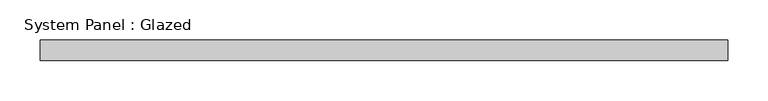
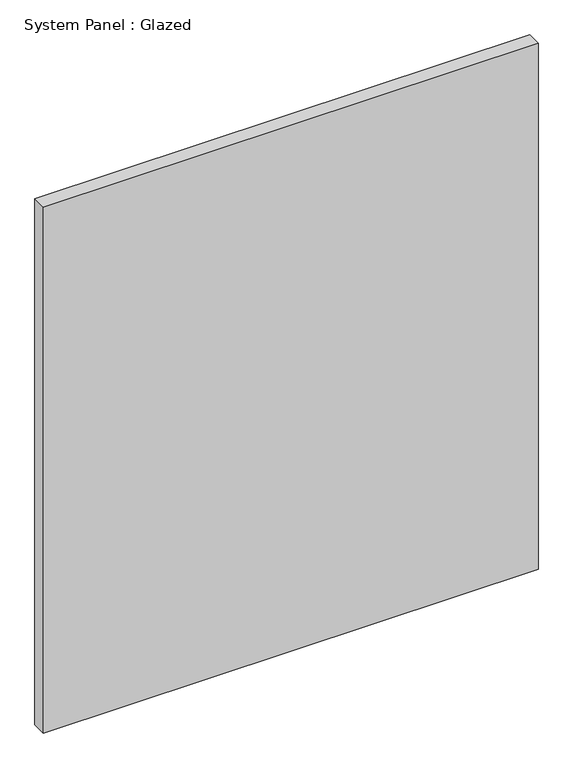
"""IFC4 building model written with IfcOpenShell, lengths in millimetres: plate geometry, System Panel : Glazed."""

from ifc_helpers import new_model, si_unit, origin, origin_with_axes, place, context, project, spatial, polyline, outline, extrude, source, transform, mapped, element, save


def system_panel_glazed_1e141fc7(model_context):
    return source(origin(), model_context, "Body", "SweptSolid", [
        extrude(outline(polyline([(425.45, 19.05), (-425.45, 19.05), (-425.45, 44.45), (425.45, 44.45), (425.45, 19.05)])), origin_with_axes(), (0.0, 0.0, 1.0), 956.453622),
    ])


if __name__ == "__main__":
    model = new_model("IFC4")
    model_context = context("Model", 3, world=origin())
    ifc_project = project(units=[si_unit("LENGTHUNIT", "METRE", prefix="MILLI")], contexts=[model_context])
    site = spatial("IfcSite", under=ifc_project)
    building = spatial("IfcBuilding", under=site)
    placement = place(None, origin())
    system_panel_glazed_shape = system_panel_glazed_1e141fc7(model_context)
    element("IfcPlate", 1, ObjectType="System Panel : Glazed", at=placement, inside=building, context=model_context, shape_type="MappedRepresentation", body=[
        mapped(system_panel_glazed_shape, transform((0.0, 0.0, 0.0), x_axis=(1.0, 0.0, 0.0), y_axis=(0.0, 1.0, 0.0), z_axis=(0.0, 0.0, 1.0))),
    ])
    save(model, "model.ifc")

# Revit data of these elements
# Type "System Panel : Glazed"
#   Construction Type Id = "GSP4R"
#   Analytic Construction = "1/8 in Pilkington single glazing"
#   Visual Light Transmittance = 0.9
#   Solar Heat Gain Coefficient = 0.86
#   Heat Transfer Coefficient (U) = 1.18115 BTU/(h·ft²·°F)
#   Define Thermal Properties by = 1
# Element 1 (IfcPlate, "System Panel : Glazed")
#   Materials on its faces: "Glass"
# Materials
#   "Glass": class "Glass", colour RGB 0 128 192, transparency 0.75, Description = "Soda Lime Glass", Cost = 0
